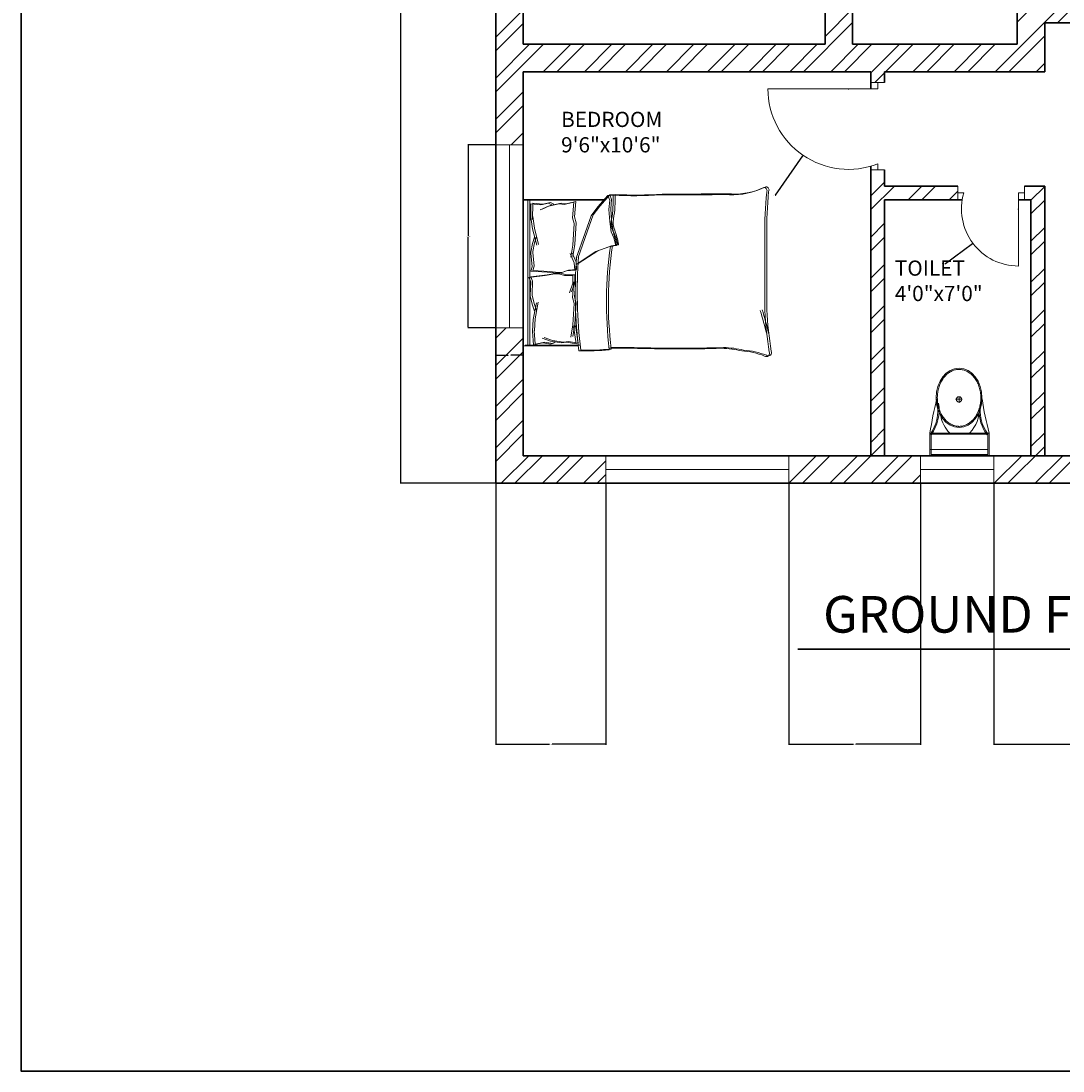
# Model space of a CAD drawing. Units: inches. Extents: x 1955 to 3324, y 980 to 3129.
# Tile 1 of 11: x 1955 to 2296, y 1704 to 2048. Entities that reach past the tile are written whole.
import ezdxf

# ---------------------------------------------------------------- set-up
doc = ezdxf.new("R2010")
doc.units = ezdxf.units.IN
for name, color, linetype, lineweight in [('A-ANNO-DIMS', 2, 'Continuous', 18), ('A-ANNO-TITL', 7, 'Continuous', 35), ('A-ANNO-TTLB', 7, 'Continuous', 35), ('A-AREA-IDEN', 7, 'Continuous', 18), ('A-DOOR', 3, 'Continuous', 18), ('A-FLOR-FIXT', 9, 'Continuous', 18), ('A-FURN', 8, 'Continuous', 18), ('A-GLAZ', 4, 'Continuous', 18), ('A-WALL', 7, 'Continuous', 35), ('A-WALL-PATT', 252, 'Continuous', 13)]:
    doc.layers.add(name, color=color, linetype=linetype, lineweight=lineweight)
doc.styles.get("Standard").update_dxf_attribs({"font": 'arial.ttf'})
doc.dimstyles.get("Standard").update_dxf_attribs({"dimtxt": 0.18, "dimasz": 0.18, "dimexe": 0.18, "dimexo": 0.0625, "dimgap": 0.09, "dimtad": 0, "dimtih": 1, "dimtoh": 1, "dimdec": 4, "dimzin": 0, "dimdsep": 46, "dimtxsty": 'Standard', "dimcen": 0.09, "dimadec": 0, "dimazin": 0, "dimtfac": 1, "dimtdec": 4, "dimtofl": 0, "dimtmove": 0, "dimatfit": 3, "dimfxl": 1, "dimtolj": 1, "dimtzin": 0, "dimarcsym": 0})

# ---------------------------------------------------------------- blocks, each defined once
blk = doc.blocks.new('A$C31115884')
for p, q in [((283.1, 497.7), (223.4, 497.7)), ((257.5, 466.4), (257.5, 523.2)), ((0, 200), (0, 0)), ((520, 200), (0, 200)), ((10, 190), (10, 10)), ((510, 190), (10, 190)), ((510, 10), (510, 190)), ((520, 0), (520, 200)), ((510, 54.5), (0, 54.5)), ((10, 10), (510, 10)), ((0, 0), (520, 0))]:
    blk.add_line(p, q)
blk.add_circle((255.6, 496.4), 23.6)
for centre, radius, start, end in [((2777.7, -204.6), 2807, 165.4549, 171.71327), ((-294.5, 403.3), 364.7, 324.20913, 9.34987), ((-294.5, 403.3), 374.7, 324.20913, 9.34987), ((805.8, 403.3), 364.7, 170.65013, 215.79087), ((3237, 905), 2807, 188.28673, 194.5451), ((139.5, 406.2), 293.5, 315.84364, 2.65635), ((805.8, 403.3), 374.7, 179.20365, 215.79087), ((383.6, 406.2), 293.5, 190.27735, 224.15636)]:
    blk.add_arc(centre, radius, start, end)
blk.add_ellipse((256.2, 509.9), major_axis=(0, -260.7), ratio=0.772727)
blk.add_open_spline([(256.2, 259.2), (263.1, 259.2), (270, 259.7), (287.8, 262.3), (298.7, 265.1), (319.9, 273.1), (330.2, 278.4), (350.1, 291.1), (359.7, 298.7), (377.7, 315.9), (386.2, 325.5), (401.7, 346.6), (408.8, 358.1), (421.3, 382.5), (426.8, 395.5), (435.9, 422.4), (439.5, 436.4), (444.8, 465.1), (446.5, 479.7), (447.9, 509.2), (447.6, 524), (445, 553.3), (442.7, 567.8), (436.3, 596), (432.1, 609.7), (421.9, 636), (416, 648.6), (402.5, 672.1), (395, 683), (378.6, 703), (369.8, 712.1), (351.1, 728), (341.3, 734.8), (320.9, 746.2), (310.4, 750.7), (288.9, 757.3), (278, 759.4), (256, 761), (245, 760.6), (223.1, 757.2), (212.3, 754.3), (191.1, 746.1), (180.8, 740.7), (160.9, 727.8), (151.4, 720.1), (133.5, 702.7), (125.1, 693), (109.6, 671.7), (102.6, 660.2), (90.2, 635.7), (84.9, 622.7), (76, 595.6), (72.4, 581.6), (67.2, 552.9), (65.6, 538.2), (64.4, 508.8), (64.8, 494), (67.5, 464.7), (69.9, 450.2), (76.6, 422), (80.8, 408.3), (91.1, 382.2), (97.2, 369.7), (110.8, 346.3), (118.4, 335.4), (134.8, 315.6), (143.7, 306.7), (162.4, 290.9), (172.3, 284.2), (192.8, 273), (203.3, 268.6), (224.8, 262.2), (235.8, 260.2), (249.9, 259.3), (253, 259.2), (256.2, 259.2)], degree=3, knots=[0, 0, 0, 0, 0.110105, 0.110105, 0.285049, 0.285049, 0.459994, 0.459994, 0.634938, 0.634938, 0.809882, 0.809882, 0.984827, 0.984827, 1.159771, 1.159771, 1.334715, 1.334715, 1.50966, 1.50966, 1.684604, 1.684604, 1.859549, 1.859549, 2.034493, 2.034493, 2.209437, 2.209437, 2.384382, 2.384382, 2.559326, 2.559326, 2.73427, 2.73427, 2.909215, 2.909215, 3.084159, 3.084159, 3.259103, 3.259103, 3.434048, 3.434048, 3.608992, 3.608992, 3.783936, 3.783936, 3.958881, 3.958881, 4.133825, 4.133825, 4.30877, 4.30877, 4.483714, 4.483714, 4.658658, 4.658658, 4.833603, 4.833603, 5.008547, 5.008547, 5.183491, 5.183491, 5.358436, 5.358436, 5.53338, 5.53338, 5.708324, 5.708324, 5.883269, 5.883269, 6.058213, 6.058213, 6.233158, 6.233158, 6.283185, 6.283185, 6.283185, 6.283185])
blk = doc.blocks.new('BED-WITH-PILLOWS')
for p, q in [((3.48, 63.33), (3.48, 81.44)), ((3.48, 63.33), (3.48, 81.44)), ((51.27, 81.44), (3.48, 81.44)), ((3.48, 79.91), (51.27, 79.91)), ((3.48, 79.91), (51.27, 79.91)), ((3.7, 62.69), (3.7, 80.8)), ((3.7, 62.69), (3.7, 80.8)), ((3.7, 79.27), (51.49, 79.27)), ((3.7, 79.27), (51.49, 79.27)), ((24.54, 78.99), (25.98, 79.57)), ((24.54, 78.99), (25.98, 79.57)), ((25.98, 79.57), (26.56, 74.22)), ((25.98, 79.57), (26.56, 74.22)), ((51.27, 81.44), (51.27, 54.83)), ((51.27, 81.44), (51.27, 54.83)), ((51.27, 81.44), (51.49, 81.44)), ((51.49, 81.44), (51.49, 80.8)), ((51.49, 80.8), (51.49, 54.19)), ((51.49, 80.8), (51.49, 54.19)), ((3.89, 78.13), (4.47, 74.95)), ((3.9, 78.11), (8.18, 78.43)), ((3.9, 78.11), (8.18, 78.43)), ((3.9, 78.13), (4.47, 74.95)), ((4.12, 77.49), (4.7, 74.31)), ((4.12, 77.49), (4.7, 74.31)), ((4.13, 77.47), (8.41, 77.8)), ((4.13, 77.47), (8.41, 77.8)), ((8.18, 78.43), (8.29, 78.42)), ((8.18, 78.43), (8.29, 78.42)), ((8.29, 78.42), (12.11, 78.13)), ((8.29, 78.42), (12.11, 78.13)), ((8.41, 77.8), (8.51, 77.78)), ((8.41, 77.8), (8.51, 77.78)), ((8.51, 77.78), (12.34, 77.49)), ((8.51, 77.78), (12.34, 77.49)), ((12.11, 78.13), (17.6, 77.12)), ((12.11, 78.13), (17.6, 77.12)), ((12.34, 77.49), (17.83, 76.48)), ((12.34, 77.49), (17.83, 76.48)), ((14.86, 77.69), (16.88, 78.42)), ((14.86, 77.69), (16.88, 78.42)), ((15.08, 77.05), (17.11, 77.78)), ((15.08, 77.05), (17.11, 77.78)), ((16.88, 78.42), (19.77, 79.14)), ((16.88, 78.42), (19.77, 79.14)), ((17.11, 77.78), (20, 78.5)), ((17.11, 77.78), (20, 78.5)), ((19.77, 79.14), (20.09, 79.14)), ((19.77, 79.14), (20.09, 79.14)), ((20, 78.5), (20.32, 78.5)), ((20, 78.5), (20.32, 78.5)), ((20.09, 79.14), (24.54, 78.99)), ((20.09, 79.14), (24.54, 78.99)), ((20.32, 78.5), (24.77, 78.36)), ((20.32, 78.5), (24.77, 78.36)), ((24.77, 78.36), (26.21, 78.93)), ((24.77, 78.36), (26.21, 78.93)), ((26.21, 78.93), (26.79, 73.58)), ((26.21, 78.93), (26.79, 73.58)), ((27.98, 78.95), (27.73, 73.58)), ((27.98, 78.95), (27.73, 73.58)), ((28.21, 78.31), (27.96, 72.94)), ((28.21, 78.31), (27.96, 72.94)), ((29.46, 78.46), (27.98, 78.95)), ((29.46, 78.46), (27.98, 78.95)), ((29.68, 77.83), (28.21, 78.31)), ((29.68, 77.83), (28.21, 78.31)), ((33.88, 78.89), (29.46, 78.46)), ((33.88, 78.89), (29.46, 78.46)), ((34.11, 78.25), (29.68, 77.83)), ((34.11, 78.25), (29.68, 77.83)), ((34.21, 78.91), (33.88, 78.89)), ((34.2, 78.91), (33.88, 78.89)), ((34.43, 78.27), (34.11, 78.25)), ((34.43, 78.27), (34.11, 78.25)), ((37.14, 78.36), (34.2, 78.91)), ((37.14, 78.36), (34.21, 78.91)), ((37.36, 77.73), (34.43, 78.27)), ((37.36, 77.73), (34.43, 78.27)), ((41.91, 78.37), (36.5, 77.02)), ((41.91, 78.37), (36.5, 77.02)), ((42.14, 77.73), (36.72, 76.38)), ((42.14, 77.73), (36.72, 76.38)), ((39.2, 77.77), (37.14, 78.36)), ((39.2, 77.77), (37.14, 78.36)), ((39.43, 77.13), (37.36, 77.73)), ((39.43, 77.13), (37.36, 77.73)), ((45.71, 78.9), (41.91, 78.37)), ((45.71, 78.9), (41.91, 78.37)), ((45.94, 78.26), (42.14, 77.73)), ((45.94, 78.26), (42.14, 77.73)), ((50.11, 78.89), (44.71, 78.98)), ((44.71, 78.98), (45.71, 78.9)), ((50.11, 78.89), (44.71, 78.98)), ((44.71, 78.98), (45.71, 78.9)), ((50.34, 78.25), (44.94, 78.34)), ((44.94, 78.34), (45.94, 78.26)), ((50.34, 78.25), (44.94, 78.34)), ((44.94, 78.34), (45.94, 78.26)), ((49.31, 73.19), (48.13, 75.86)), ((49.31, 73.19), (48.13, 75.86)), ((50.11, 78.89), (49.73, 75.68)), ((50.11, 78.89), (49.73, 75.68)), ((50.34, 78.25), (49.96, 75.04)), ((50.34, 78.25), (49.96, 75.04)), ((4.47, 74.95), (4.04, 72.34)), ((4.47, 74.95), (4.04, 72.34)), ((4.04, 72.34), (4.62, 71.33)), ((4.04, 72.34), (4.62, 71.33)), ((4.7, 74.31), (4.27, 71.7)), ((4.7, 74.31), (4.27, 71.7)), ((4.47, 68.87), (5.05, 72.49)), ((4.47, 68.87), (5.05, 72.49)), ((5.05, 72.49), (6.06, 75.24)), ((5.05, 72.49), (6.06, 75.24)), ((5.28, 71.85), (6.29, 74.6)), ((5.28, 71.85), (6.29, 74.6)), ((26.56, 74.22), (27.14, 71.04)), ((26.56, 74.22), (27.14, 71.04)), ((26.79, 73.58), (27.37, 70.4)), ((26.79, 73.58), (27.37, 70.4)), ((27.73, 73.58), (27.36, 70.37)), ((27.73, 73.58), (27.36, 70.37)), ((27.96, 72.94), (27.58, 69.73)), ((27.96, 72.94), (27.58, 69.73)), ((49.54, 72.55), (48.36, 75.23)), ((49.54, 72.55), (48.36, 75.23)), ((50.11, 69.61), (49.31, 73.19)), ((50.11, 69.61), (49.31, 73.19)), ((50.34, 68.98), (49.54, 72.55)), ((50.34, 68.98), (49.54, 72.55)), ((49.73, 75.68), (50.33, 73.11)), ((49.73, 75.68), (50.33, 73.11)), ((50.33, 73.11), (49.81, 72.06)), ((50.33, 73.11), (49.82, 72.06)), ((49.96, 75.04), (50.56, 72.47)), ((49.96, 75.04), (50.56, 72.47)), ((50.56, 72.47), (50.04, 71.42)), ((50.56, 72.47), (50.04, 71.42)), ((4.27, 71.7), (4.85, 70.69)), ((4.27, 71.7), (4.85, 70.69)), ((4.7, 68.23), (5.28, 71.85)), ((4.7, 68.23), (5.28, 71.85)), ((27.14, 69.74), (26.56, 67.86)), ((27.14, 69.74), (26.56, 67.86)), ((27.37, 69.1), (26.79, 67.22)), ((27.37, 69.1), (26.79, 67.22)), ((27.14, 71.04), (27.14, 69.74)), ((27.14, 71.04), (27.14, 69.74)), ((27.36, 70.37), (27.44, 69.07)), ((27.36, 70.37), (27.44, 69.07)), ((27.37, 70.4), (27.37, 69.1)), ((27.37, 70.4), (27.37, 69.1)), ((27.44, 69.07), (28.13, 67.23)), ((27.44, 69.07), (28.13, 67.23)), ((27.58, 69.73), (27.66, 68.43)), ((27.58, 69.73), (27.66, 68.43)), ((49.92, 68.01), (50.11, 69.61)), ((49.92, 68.01), (50.11, 69.61)), ((50.15, 67.37), (50.34, 68.98)), ((50.15, 67.37), (50.34, 68.98)), ((4.18, 64.1), (4.76, 67.28)), ((4.18, 64.1), (4.76, 67.28)), ((4.41, 63.46), (4.99, 66.64)), ((4.41, 63.46), (4.99, 66.64)), ((4.76, 67.28), (4.47, 68.87)), ((4.76, 67.28), (4.47, 68.87)), ((4.99, 66.64), (4.7, 68.23)), ((4.99, 66.64), (4.7, 68.23)), ((6.38, 65.81), (10.41, 65.15)), ((6.38, 65.81), (10.41, 65.15)), ((24.1, 65.18), (20.96, 66.27)), ((24.1, 65.18), (20.96, 66.27)), ((24.33, 64.54), (21.19, 65.63)), ((24.33, 64.54), (21.19, 65.63)), ((26.56, 67.86), (26.56, 65.18)), ((26.56, 67.86), (26.56, 65.18)), ((26.79, 67.22), (26.79, 64.54)), ((26.79, 67.22), (26.79, 64.54)), ((27.66, 68.43), (28.36, 66.59)), ((27.66, 68.43), (28.36, 66.59)), ((28.13, 67.23), (28.3, 64.55)), ((28.13, 67.23), (28.3, 64.55)), ((28.36, 66.59), (28.53, 63.91)), ((28.36, 66.59), (28.53, 63.91)), ((30.75, 64.7), (33.82, 65.99)), ((30.75, 64.7), (33.82, 65.99)), ((32.56, 65.81), (36.6, 65.15)), ((32.56, 65.81), (36.6, 65.15)), ((50.7, 64.87), (49.92, 68.01)), ((50.7, 64.87), (49.92, 68.01)), ((50.93, 64.23), (50.15, 67.37)), ((50.93, 64.23), (50.15, 67.37)), ((9.28, 64.83), (4.18, 64.1)), ((9.28, 64.83), (4.18, 64.1)), ((9.51, 64.19), (4.41, 63.46)), ((9.51, 64.19), (4.41, 63.46)), ((6.61, 65.18), (10.64, 64.51)), ((6.61, 65.18), (10.64, 64.51)), ((10.41, 65.15), (9.28, 64.83)), ((10.41, 65.15), (9.28, 64.83)), ((10.64, 64.51), (9.51, 64.19)), ((10.64, 64.51), (9.51, 64.19)), ((10.41, 65.15), (17.42, 64.72)), ((10.41, 65.15), (17.42, 64.72)), ((10.64, 64.51), (17.65, 64.08)), ((10.64, 64.51), (17.65, 64.08)), ((17.42, 64.72), (19.38, 65.27)), ((17.42, 64.72), (19.38, 65.27)), ((17.65, 64.08), (19.61, 64.63)), ((17.65, 64.08), (19.61, 64.63)), ((19.38, 65.27), (24.52, 64.87)), ((19.38, 65.27), (24.52, 64.87)), ((19.61, 64.63), (24.74, 64.23)), ((19.61, 64.63), (24.74, 64.23)), ((26.56, 65.18), (24.1, 65.18)), ((26.56, 65.18), (24.1, 65.18)), ((26.79, 64.54), (24.33, 64.54)), ((26.79, 64.54), (24.33, 64.54)), ((28.3, 64.55), (30.75, 64.7)), ((28.3, 64.55), (30.75, 64.7)), ((28.53, 63.91), (30.98, 64.06)), ((28.53, 63.91), (30.98, 64.06)), ((30.26, 64.06), (34.45, 57.57)), ((30.26, 64.06), (34.45, 57.57)), ((30.49, 63.42), (34.68, 56.93)), ((30.49, 63.42), (34.68, 56.93)), ((30.98, 64.06), (34.05, 65.35)), ((30.98, 64.06), (34.05, 65.35)), ((40.64, 61.13), (32.31, 64.06)), ((40.64, 61.13), (32.31, 64.06)), ((40.87, 60.49), (32.53, 63.42)), ((40.87, 60.49), (32.54, 63.42)), ((32.79, 65.18), (36.83, 64.51)), ((32.79, 65.18), (36.82, 64.51)), ((36.6, 65.15), (43.61, 64.72)), ((36.6, 65.15), (43.61, 64.72)), ((36.82, 64.51), (43.83, 64.08)), ((36.83, 64.51), (43.84, 64.08)), ((43.61, 64.72), (45.57, 65.27)), ((43.61, 64.72), (45.57, 65.27)), ((43.83, 64.08), (45.8, 64.63)), ((43.84, 64.08), (45.8, 64.63)), ((45.57, 65.27), (50.7, 64.87)), ((45.57, 65.27), (50.7, 64.87)), ((45.8, 64.63), (50.93, 64.23)), ((45.8, 64.63), (50.93, 64.23)), ((46.22, 59.11), (40.64, 61.13)), ((46.22, 59.11), (40.64, 61.13)), ((46.45, 58.48), (40.87, 60.49)), ((46.45, 58.48), (40.87, 60.49)), ((49.16, 56.95), (46.22, 59.11)), ((49.16, 56.95), (46.22, 59.11)), ((34.45, 57.57), (36.15, 53.08)), ((34.45, 57.57), (36.15, 53.08)), ((34.68, 56.93), (36.38, 52.44)), ((34.68, 56.93), (36.38, 52.44)), ((49.39, 56.31), (46.45, 58.48)), ((49.39, 56.31), (46.45, 58.48)), ((52.87, 53.7), (49.16, 56.95)), ((52.87, 53.7), (49.16, 56.95)), ((53.1, 53.06), (49.39, 56.31)), ((53.1, 53.06), (49.39, 56.31)), ((36.15, 53.08), (36.46, 51.07)), ((36.15, 53.08), (36.46, 51.07)), ((36.38, 52.44), (36.69, 50.43)), ((36.38, 52.44), (36.69, 50.43)), ((36.46, 51.07), (38.94, 51.69)), ((36.46, 51.07), (38.94, 51.69)), ((38.94, 51.69), (40.95, 52.61)), ((38.94, 51.69), (40.95, 52.61)), ((39.17, 51.05), (41.18, 51.97)), ((39.17, 51.05), (41.18, 51.97)), ((40.95, 52.61), (44.36, 53.08)), ((40.95, 52.61), (44.36, 53.08)), ((41.18, 51.97), (44.59, 52.44)), ((41.18, 51.97), (44.59, 52.44)), ((44.36, 53.08), (48.23, 53.39)), ((44.36, 53.08), (48.23, 53.39)), ((44.59, 52.44), (48.46, 52.75)), ((44.59, 52.44), (48.46, 52.75)), ((48.23, 53.39), (51.33, 53.08)), ((48.23, 53.39), (51.33, 53.08)), ((48.46, 52.75), (51.56, 52.44)), ((48.46, 52.75), (51.56, 52.44)), ((51.33, 53.08), (52.87, 53.7)), ((51.33, 53.08), (52.87, 53.7)), ((51.56, 52.44), (53.1, 53.06)), ((51.56, 52.44), (53.1, 53.06)), ((52.95, 51.95), (52.87, 53.7, 3.87)), ((52.95, 51.95), (52.87, 53.7, 3.87)), ((53.18, 51.31), (53.1, 53.06, 3.87)), ((53.18, 51.31), (53.1, 53.06, 3.87)), ((36.69, 50.43), (39.17, 51.05)), ((36.69, 50.43), (39.17, 51.05)), ((15.06, 2.2), (39.68, 2.2)), ((15.06, 2.2), (39.68, 2.2)), ((15.29, 1.56), (39.91, 1.56)), ((15.29, 1.56), (39.91, 1.56))]:
    blk.add_line(p, q)
for centre, radius, start, end in [((85.16, 61.35), 83.31, 178.7218, 185.604), ((85.16, 61.35), 83.31, 178.7218, 185.604), ((21.36, -100.61), 164.97, 86.0865, 96.7821), ((21.36, -100.61), 164.97, 86.0865, 96.7821), ((85.39, 60.71), 83.31, 178.7218, 185.604), ((85.39, 60.71), 83.31, 178.7218, 185.604), ((21.59, -101.25), 164.97, 86.0865, 96.7821), ((21.59, -101.25), 164.97, 86.0865, 96.7821), ((17.76, -74.87), 129.02, 81.7845, 96.9006), ((17.76, -74.87), 129.02, 81.7845, 96.9006), ((17.98, -75.51), 129.02, 81.7845, 96.9006), ((17.98, -75.51), 129.02, 81.7845, 96.9006), ((-167.31, 50.27), 170.11, 358.4762, 1.0082), ((-167.31, 50.27), 170.11, 358.4762, 1.0082), ((-167.08, 49.63), 170.11, 358.4762, 1.0082), ((-167.08, 49.63), 170.11, 358.4762, 1.0082), ((31.15, 79.96), 29.65, 280.6617, 289.8806), ((31.15, 79.96), 29.65, 280.6617, 289.8806), ((43.74, 46.38), 6.22, 78.6608, 113.7384), ((43.74, 46.38), 6.22, 78.6608, 113.7384), ((43.97, 45.74), 6.22, 78.6608, 113.7384), ((43.97, 45.74), 6.22, 78.6608, 113.7384), ((51.33, 88.1), 36.18, 259.8763, 272.5657), ((51.33, 88.1), 36.18, 259.8763, 272.5657), ((51.56, 87.46), 36.18, 259.8763, 272.5657), ((51.56, 87.46), 36.18, 259.8763, 272.5657), ((182.27, 45.13), 129.5, 176.9791, 183.8365), ((182.27, 45.13), 129.5, 176.9791, 183.8365), ((36.64, 51), 0.185, 160.2464, 271.1377), ((36.64, 51), 0.185, 160.2464, 271.1377), ((36.87, 50.36), 0.185, 160.2464, 271.1377), ((36.86, 50.36), 0.185, 160.2464, 271.1377), ((31.38, 79.32), 29.65, 280.6617, 289.8806), ((31.38, 79.32), 29.65, 280.6617, 289.8806), ((182.49, 44.49), 129.5, 176.9791, 183.8365), ((182.49, 44.49), 129.5, 176.9791, 183.8365), ((484.82, 30.83), 482.31, 178.2277, 181.7185), ((484.82, 30.83), 482.31, 178.2277, 181.7185), ((485.05, 30.19), 482.31, 178.2277, 181.7185), ((485.05, 30.19), 482.31, 178.2277, 181.7185), ((-4508.74, 13.62), 4561.86, 0.00217, 0.28689), ((-4508.74, 13.62), 4561.86, 0.00217, 0.28689), ((-4508.51, 12.98), 4561.86, 0.00217, 0.28689), ((-4508.51, 12.98), 4561.86, 0.00217, 0.28689), ((-26.9, 16.93), 29.63, 346.0648, 358.9113), ((-26.9, 16.93), 29.63, 346.0648, 358.9113), ((-26.67, 16.29), 29.63, 346.0648, 358.9113), ((-26.67, 16.29), 29.63, 346.0648, 358.9113), ((76.16, 12.78), 23.07, 177.4714, 206.4681), ((76.16, 12.78), 23.07, 177.4714, 206.4681), ((76.39, 12.14), 23.07, 177.4714, 206.4681), ((76.39, 12.14), 23.07, 177.4714, 206.4681), ((-21.66, 11.17), 23.56, 337.9751, 356.652), ((-21.66, 11.17), 23.56, 337.9751, 356.652), ((-21.43, 10.53), 23.56, 337.9751, 356.652), ((-21.43, 10.53), 23.56, 337.9751, 356.652), ((-17.22, 105.16), 106.46, 283.3832, 287.7053), ((-17.22, 105.16), 106.46, 283.3832, 287.7053), ((1.09, 1.73), 1.09, 146.1736, 293.4781), ((1.09, 1.73), 1.09, 146.1736, 293.4781), ((1.32, 1.09), 1.09, 146.1736, 293.4781), ((1.32, 1.09), 1.09, 146.1736, 293.4781), ((21.43, -119.39), 121.76, 92.9958, 99.4091), ((21.43, -119.39), 121.76, 92.9958, 99.4091), ((21.66, -120.03), 121.76, 92.9958, 99.4091), ((21.66, -120.03), 121.76, 92.9958, 99.4091), ((-16.99, 104.52), 106.46, 283.3832, 287.7053), ((-16.99, 104.52), 106.46, 283.3832, 287.7053), ((41.15, -130.83), 133.04, 84.4998, 90.6351), ((41.15, -130.83), 133.04, 84.4998, 90.6351), ((41.38, -131.47), 133.04, 84.4998, 90.6351), ((41.38, -131.47), 133.04, 84.4998, 90.6351), ((54.41, 2.57), 1.1, 242.6588, 356.02), ((54.41, 2.57), 1.1, 242.6588, 356.02), ((54.64, 1.93), 1.1, 242.6588, 356.02), ((54.64, 1.93), 1.1, 242.6588, 356.02)]:
    blk.add_arc(centre, radius, start, end)
blk = doc.blocks.new('DOOR-BED-S')
for p, q in [((38.25, 28.66), (33.75, 28.66)), ((33.75, 28.66), (36, 28.66)), ((36, 28.66), (36, 26.66)), ((36, 26.66), (0, 26.66)), ((36, 0), (36, 2)), ((33.75, 0), (38.25, 0)), ((38.25, 0), (36, 0))]:
    blk.add_line(p, q)
blk.add_arc((26.45, 26.66), 26.45, 180, 291.1718)
blk = doc.blocks.new('DOOR-WC-S')
for p, q in [((0, 21.75), (0, 26.25)), ((0, 26.25), (0, 24)), ((21.9, 21.75), (21.9, 26.25)), ((21.9, 26.25), (21.9, 24)), ((0, 24), (2, 24)), ((21.9, 24), (19.9, 24)), ((19.9, 24), (19.9, 0))]:
    blk.add_line(p, q)
blk.add_arc((19.9, 18.68), 18.68, 163.4391, 270)
blk = doc.blocks.new('WIN-PLAN-60-A')
for p, q in [((0, 60), (9, 60)), ((9, 60), (4.5, 60)), ((4.5, 60), (4.5, 0)), ((4.5, 0), (0, 0)), ((0, 0), (9, 0))]:
    blk.add_line(p, q)
blk = doc.blocks.new('WIN-PLAN-60-B')
for p, q in [((0, 0), (0, 9)), ((0, 9), (0, 4.5)), ((60, 4.5), (60, 9)), ((60, 9), (60, 0)), ((0, 4.5), (60, 4.5))]:
    blk.add_line(p, q)
blk = doc.blocks.new('WIN-PLAN-24-A')
for p, q in [((0, 9), (0, 0)), ((24, 4.5), (24, 9)), ((24, 9), (24, 0)), ((0, 0), (0, 4.5)), ((0, 4.5), (24, 4.5))]:
    blk.add_line(p, q)
blk = doc.blocks.new('*D33')
at = {"layer": 'A-ANNO-DIMS', "color": 0, "lineweight": -2, "transparency": 16777216}
for p, q in [((2110.15, 2007.51), (2101.03, 2007.51)), ((2101.21, 2007.33), (2101.21, 1977.7)), ((2101.21, 1947.69), (2101.21, 1977.33)), ((2110.15, 1947.51), (2101.03, 1947.51))]:
    blk.add_line(p, q, dxfattribs=at)
at = {"layer": 'A-ANNO-DIMS', "color": 0, "transparency": 16777216}
for points in [[(2101.18, 2007.33), (2101.24, 2007.33), (2101.21, 2007.51)], [(2101.18, 1947.69), (2101.24, 1947.69), (2101.21, 1947.51)]]:
    blk.add_solid(points, dxfattribs=at)
at = {"layer": 'Defpoints', "color": 0, "transparency": 16777216}
for p in [(2110.21, 2007.51), (2101.21, 1947.51), (2110.21, 1947.51)]:
    blk.add_point(p, dxfattribs=at)
at = {"layer": 'A-ANNO-DIMS', "color": 0, "transparency": 16777216, "insert": (2101.21, 1977.51), "char_height": 0.18, "attachment_point": 5}
blk.add_mtext('\\A1;WIN. 60 TYP.', dxfattribs=at)
blk = doc.blocks.new('*D34')
at = {"layer": 'A-ANNO-DIMS', "color": 0, "lineweight": -2, "transparency": 16777216}
for p, q in [((2110.21, 1947.45), (2110.21, 1938.33)), ((2119.21, 1947.45), (2119.21, 1938.33)), ((2110.39, 1938.51), (2114.25, 1938.51)), ((2119.03, 1938.51), (2115.17, 1938.51))]:
    blk.add_line(p, q, dxfattribs=at)
at = {"layer": 'A-ANNO-DIMS', "color": 0, "transparency": 16777216}
for points in [[(2110.39, 1938.54), (2110.39, 1938.48), (2110.21, 1938.51)], [(2119.03, 1938.54), (2119.03, 1938.48), (2119.21, 1938.51)]]:
    blk.add_solid(points, dxfattribs=at)
at = {"layer": 'Defpoints', "color": 0, "transparency": 16777216}
for p in [(2110.21, 1947.51), (2119.21, 1947.51), (2119.21, 1938.51)]:
    blk.add_point(p, dxfattribs=at)
at = {"layer": 'A-ANNO-DIMS', "color": 0, "transparency": 16777216, "insert": (2114.71, 1938.51), "char_height": 0.18, "attachment_point": 5}
blk.add_mtext('\\A1;9 TYP.', dxfattribs=at)
blk = doc.blocks.new('*D92')
at = {"layer": 'A-ANNO-DIMS', "color": 0, "lineweight": -2, "transparency": 16777216}
for p, q in [((2110.15, 2456.5), (2078.88, 2456.5)), ((2079.06, 2456.32), (2079.06, 2176.69)), ((2079.06, 1896.68), (2079.06, 2176.32)), ((2110.15, 1896.5), (2078.88, 1896.5))]:
    blk.add_line(p, q, dxfattribs=at)
at = {"layer": 'A-ANNO-DIMS', "color": 0, "transparency": 16777216}
for points in [[(2079.03, 2456.32), (2079.09, 2456.32), (2079.06, 2456.5)], [(2079.03, 1896.68), (2079.09, 1896.68), (2079.06, 1896.5)]]:
    blk.add_solid(points, dxfattribs=at)
at = {"layer": 'Defpoints', "color": 0, "transparency": 16777216}
for p in [(2079.06, 2456.5), (2110.21, 2456.5), (2110.21, 1896.5)]:
    blk.add_point(p, dxfattribs=at)
at = {"layer": 'A-ANNO-DIMS', "color": 0, "transparency": 16777216, "insert": (2079.06, 2176.5), "char_height": 0.18, "attachment_point": 5}
blk.add_mtext('\\A1;560', dxfattribs=at)
blk = doc.blocks.new('*D107')
at = {"layer": 'A-ANNO-DIMS', "color": 0, "lineweight": -2, "transparency": 16777216}
for p, q in [((2110.21, 1896.44), (2110.21, 1810.7)), ((2146.36, 1896.44), (2146.36, 1810.7)), ((2110.39, 1810.88), (2127.89, 1810.88)), ((2146.18, 1810.88), (2128.68, 1810.88))]:
    blk.add_line(p, q, dxfattribs=at)
at = {"layer": 'A-ANNO-DIMS', "color": 0, "transparency": 16777216}
for points in [[(2110.39, 1810.91), (2110.39, 1810.85), (2110.21, 1810.88)], [(2146.18, 1810.91), (2146.18, 1810.85), (2146.36, 1810.88)]]:
    blk.add_solid(points, dxfattribs=at)
at = {"layer": 'Defpoints', "color": 0, "transparency": 16777216}
for p in [(2110.21, 1896.5), (2146.36, 1896.5), (2146.36, 1810.88)]:
    blk.add_point(p, dxfattribs=at)
at = {"layer": 'A-ANNO-DIMS', "color": 0, "transparency": 16777216, "insert": (2128.29, 1810.88), "char_height": 0.18, "attachment_point": 5}
blk.add_mtext('\\A1;36.15', dxfattribs=at)
blk = doc.blocks.new('*D108')
at = {"layer": 'A-ANNO-DIMS', "color": 0, "lineweight": -2, "transparency": 16777216}
for p, q in [((2206.36, 1896.44), (2206.36, 1810.7)), ((2249.49, 1896.44), (2249.49, 1810.7)), ((2206.54, 1810.88), (2227.53, 1810.88)), ((2249.31, 1810.88), (2228.32, 1810.88))]:
    blk.add_line(p, q, dxfattribs=at)
at = {"layer": 'A-ANNO-DIMS', "color": 0, "transparency": 16777216}
for points in [[(2206.54, 1810.91), (2206.54, 1810.85), (2206.36, 1810.88)], [(2249.31, 1810.91), (2249.31, 1810.85), (2249.49, 1810.88)]]:
    blk.add_solid(points, dxfattribs=at)
at = {"layer": 'Defpoints', "color": 0, "transparency": 16777216}
for p in [(2206.36, 1896.5), (2249.49, 1896.5), (2249.49, 1810.88)]:
    blk.add_point(p, dxfattribs=at)
at = {"layer": 'A-ANNO-DIMS', "color": 0, "transparency": 16777216, "insert": (2227.93, 1810.88), "char_height": 0.18, "attachment_point": 5}
blk.add_mtext('\\A1;43.13', dxfattribs=at)
blk = doc.blocks.new('*D109')
at = {"layer": 'A-ANNO-DIMS', "color": 0, "lineweight": -2, "transparency": 16777216}
for p, q in [((2273.49, 1896.44), (2273.49, 1810.7)), ((2342.7, 1896.44), (2342.7, 1810.7)), ((2273.67, 1810.88), (2307.72, 1810.88)), ((2342.52, 1810.88), (2308.47, 1810.88))]:
    blk.add_line(p, q, dxfattribs=at)
at = {"layer": 'A-ANNO-DIMS', "color": 0, "transparency": 16777216}
for points in [[(2273.67, 1810.91), (2273.67, 1810.85), (2273.49, 1810.88)], [(2342.52, 1810.91), (2342.52, 1810.85), (2342.7, 1810.88)]]:
    blk.add_solid(points, dxfattribs=at)
at = {"layer": 'Defpoints', "color": 0, "transparency": 16777216}
for p in [(2273.49, 1896.5), (2342.7, 1896.5), (2342.7, 1810.88)]:
    blk.add_point(p, dxfattribs=at)
at = {"layer": 'A-ANNO-DIMS', "color": 0, "transparency": 16777216, "insert": (2308.09, 1810.88), "char_height": 0.18, "attachment_point": 5}
blk.add_mtext('\\A1;69.21', dxfattribs=at)
blk = doc.blocks.new('*D144')
at = {"layer": 'A-ANNO-DIMS', "color": 0, "lineweight": -2, "transparency": 16777216}
for p, q in [((2225.82, 2025.93), (2226, 2025.93)), ((2225.91, 2025.84), (2225.91, 2026.02)), ((2201.99, 1991.02), (2210.86, 2003.96)), ((2201.81, 1991.02), (2201.99, 1991.02))]:
    blk.add_line(p, q, dxfattribs=at)
at = {"layer": 'A-ANNO-DIMS', "color": 0, "transparency": 16777216}
blk.add_solid([(2210.83, 2003.98), (2210.88, 2003.94), (2210.96, 2004.11)], dxfattribs=at)
at = {"layer": 'Defpoints', "color": 0, "transparency": 16777216}
for p in [(2225.91, 2025.93), (2210.96, 2004.11)]:
    blk.add_point(p, dxfattribs=at)
at = {"layer": 'A-ANNO-DIMS', "color": 0, "transparency": 16777216, "insert": (2201.33, 1991.02), "char_height": 0.18, "attachment_point": 5}
blk.add_mtext('\\A1;R26.45', dxfattribs=at)
blk = doc.blocks.new('*D146')
at = {"layer": 'A-ANNO-DIMS', "color": 0, "lineweight": -2, "transparency": 16777216}
for p, q in [((2281.52, 1986.43), (2281.7, 1986.43)), ((2281.61, 1986.34), (2281.61, 1986.52)), ((2257.66, 1968.56), (2266.5, 1975.16)), ((2257.48, 1968.56), (2257.66, 1968.56))]:
    blk.add_line(p, q, dxfattribs=at)
at = {"layer": 'A-ANNO-DIMS', "color": 0, "transparency": 16777216}
blk.add_solid([(2266.48, 1975.18), (2266.51, 1975.13), (2266.64, 1975.26)], dxfattribs=at)
at = {"layer": 'Defpoints', "color": 0, "transparency": 16777216}
for p in [(2281.61, 1986.43), (2266.64, 1975.26)]:
    blk.add_point(p, dxfattribs=at)
at = {"layer": 'A-ANNO-DIMS', "color": 0, "transparency": 16777216, "insert": (2256.93, 1968.56), "char_height": 0.18, "attachment_point": 5}
blk.add_mtext('\\A1;R18.677', dxfattribs=at)

msp = doc.modelspace()

# ---------------------------------------------------------------- hatches: boundary and pattern name
at = {"layer": 'A-WALL-PATT'}
h = msp.add_hatch(dxfattribs=at)
h.set_pattern_fill('ANSI32', color=256)
h.paths.add_polyline_path([(2361.4775, 2456.5037), (2270.2755, 2456.5037), (2270.2755, 2447.5037), (2285.7102, 2447.5037), (2285.7102, 2363.5037), (2281.1795, 2363.5037), (2281.1795, 2359.0037), (2290.2102, 2359.0037), (2290.2102, 2447.5037), (2361.4775, 2447.5037), (2361.4775, 2452.0037)])
h.paths.add_polyline_path([(2246.2755, 2456.5037), (2197.6809, 2456.5037), (2197.6809, 2447.5037), (2233.2102, 2447.5037), (2233.2102, 2355.6044), (2237.7102, 2355.6044), (2237.7102, 2447.5037), (2246.2755, 2447.5037)], flags=17)
h.paths.add_polyline_path([(2137.6809, 2456.5037), (2110.2102, 2456.5037), (2110.2102, 2312.5037), (2152.2102, 2312.5037), (2281.2102, 2312.5037), (2281.2102, 2107.6185), (2290.2102, 2107.6185), (2290.2102, 2267.9289), (2329.216, 2267.9289), (2329.216, 2272.4289), (2329.216, 2276.9289), (2290.2102, 2276.9289), (2290.2102, 2321.5037), (2281.2102, 2321.5037), (2119.2102, 2321.5037), (2119.2102, 2447.5037), (2137.6809, 2447.5037)])
h.paths.add_polyline_path([(2515.2102, 2456.5037), (2421.4775, 2456.5037), (2421.4775, 2447.5037), (2506.2102, 2447.5037), (2506.2102, 2415.6626), (2515.2102, 2415.6626)])
h.paths.add_polyline_path([(2515.2102, 2355.6626), (2506.2102, 2355.6626), (2506.2102, 2321.5037), (2424.9282, 2321.5037), (2424.9282, 2312.5037), (2461.2102, 2312.5037), (2470.2102, 2312.5037), (2515.2102, 2312.5037)])
h.paths.add_polyline_path([(2515.2102, 2232.5037), (2470.2102, 2232.5037), (2470.2102, 2237.3759), (2465.7102, 2237.3759), (2461.2102, 2237.3759), (2461.2102, 2232.5037), (2377.2219, 2232.5037), (2377.2219, 2321.5037), (2368.2219, 2321.5037), (2368.2219, 2276.9289), (2359.3802, 2276.9289), (2359.3802, 2272.4289), (2359.3802, 2267.9289), (2368.2219, 2267.9289), (2368.2219, 2223.5037), (2377.2219, 2223.5037), (2461.2102, 2223.5037), (2506.2102, 2223.5037), (2506.2102, 2129.5037), (2461.2102, 2129.5037), (2387.2102, 2129.5037), (2368.2219, 2129.5037), (2368.2219, 2056.4936), (2361.0095, 2056.4936), (2361.0095, 2051.9936), (2361.0095, 2047.4936), (2368.2219, 2047.4936), (2368.2219, 2031.5037), (2377.2219, 2031.5037), (2377.2219, 2120.5037), (2461.2102, 2120.5037), (2461.2102, 2112.7921), (2470.2102, 2112.7921), (2470.2102, 2120.5037), (2515.2102, 2120.5037), (2515.2102, 2129.5037)])
h.paths.add_polyline_path([(2470.2102, 2277.1758), (2461.2102, 2277.1758), (2461.2102, 2272.5037), (2461.2102, 2270.2549), (2470.2102, 2270.2549), (2470.2102, 2272.5037)], flags=17)
h.paths.add_polyline_path([(2515.2102, 2040.5037), (2470.2102, 2040.5037), (2417.8264, 2040.5037), (2417.8264, 2031.5037), (2506.2102, 2031.5037), (2506.2102, 2005.3639), (2515.2102, 2005.3639)])
h.paths.add_polyline_path([(2506.2102, 1905.5037), (2402.6963, 1905.5037), (2402.6963, 1896.5037), (2506.2102, 1896.5037)])
h.paths.add_polyline_path([(2515.2102, 1945.3639), (2506.2102, 1945.3639), (2506.2102, 1905.5037), (2506.2102, 1896.5037), (2515.2102, 1896.5037)])
h.paths.add_polyline_path([(2342.6963, 1901.0037), (2342.6963, 1905.5037), (2273.4892, 1905.5037), (2273.4892, 1896.5037), (2342.6963, 1896.5037)])
h.paths.add_polyline_path([(2290.2102, 1994.0037), (2283.612, 1994.0037), (2283.612, 1991.7537), (2283.612, 1989.5037), (2285.7102, 1989.5037), (2285.7102, 1905.5037), (2290.2102, 1905.5037)])
h.paths.add_polyline_path([(2249.4892, 1905.5037), (2237.7102, 1905.5037), (2206.3617, 1905.5037), (2206.3617, 1896.5037), (2249.4892, 1896.5037), (2249.4892, 1901.0037)])
h.paths.add_polyline_path([(2237.7102, 1989.5037), (2261.7102, 1989.5037), (2261.7102, 1994.0037), (2237.7102, 1994.0037), (2237.7102, 1999.266), (2235.4602, 1999.266), (2233.2102, 1999.266), (2233.2102, 1994.0037), (2233.2102, 1905.5037), (2237.7102, 1905.5037)])
h.paths.add_polyline_path([(2119.2102, 1947.5144), (2110.2102, 1947.5144), (2110.2102, 1896.5037), (2119.2102, 1896.5037), (2146.3617, 1896.5037), (2146.3617, 1901.0037), (2146.3617, 1905.5037), (2119.2102, 1905.5037)])
h.paths.add_polyline_path([(2119.2102, 2068.6379), (2110.2102, 2068.6379), (2110.2102, 2007.5144), (2119.2102, 2007.5144), (2119.2102, 2031.5037), (2233.2102, 2031.5037), (2233.2102, 2027.9287), (2235.4602, 2027.9287), (2237.7102, 2027.9287), (2237.7102, 2031.5037), (2281.2102, 2031.5037), (2290.2102, 2031.5037), (2290.2102, 2047.4936), (2326.409, 2047.4936), (2326.409, 2056.4936), (2290.2102, 2056.4936), (2290.2102, 2071.2722), (2285.7102, 2071.2722), (2281.2102, 2071.2722), (2281.2102, 2040.5037), (2227.2102, 2040.5037), (2227.2102, 2111.2571), (2222.7102, 2111.2571), (2218.2102, 2111.2571), (2218.2102, 2040.5037), (2119.2102, 2040.5037)])
h.paths.add_polyline_path([(2236.9166, 2214.5037), (2161.2102, 2214.5037), (2161.2102, 2221.6488), (2152.2102, 2221.6488), (2152.2102, 2214.5037), (2110.2102, 2214.5037), (2110.2102, 2205.5037), (2131.2394, 2205.5037), (2131.2394, 2198.3478), (2140.2394, 2198.3478), (2140.2394, 2205.5037), (2224.2394, 2205.5037), (2224.2394, 2200.2317), (2228.7394, 2200.2317), (2233.2394, 2200.2317), (2233.2394, 2205.5037), (2236.9166, 2205.5037)], flags=17)
h.paths.add_polyline_path([(2236.9166, 2157.5037), (2233.2394, 2157.5037), (2233.2394, 2178.9172), (2228.7394, 2178.9172), (2224.2394, 2178.9172), (2224.2394, 2157.5037), (2140.2394, 2157.5037), (2140.2394, 2174.3478), (2131.2394, 2174.3478), (2131.2394, 2157.5037), (2110.2102, 2157.5037), (2110.2102, 2128.6379), (2119.2102, 2128.6379), (2119.2102, 2148.5037), (2218.2102, 2148.5037), (2218.2102, 2141.7262), (2222.7102, 2141.7262), (2227.2102, 2141.7262), (2227.2102, 2148.5037), (2236.9166, 2148.5037)], flags=0)
h.paths.add_polyline_path([(3084.7449, 2537.3808), (3212.7954, 2537.3808), (3212.7954, 2555.9271), (3084.7449, 2555.9271)], flags=9)
h.paths.add_polyline_path([(3068.7485, 2853.43), (3169.977, 2853.43), (3169.977, 2871.9764), (3068.7485, 2871.9764)], flags=9)
h.paths.add_polyline_path([(3074.1798, 2918.0252), (3126.4732, 2918.0252), (3126.4732, 2936.5716), (3074.1798, 2936.5716)], flags=9)
h.paths.add_polyline_path([(3073.0928, 2947.3127), (3199.0499, 2947.3127), (3199.0499, 2965.8591), (3073.0928, 2965.8591)], flags=9)
h.paths.add_polyline_path([(2733.8393, 2484.8678), (2879.7915, 2484.8678), (2879.7915, 2521.9606), (2733.8393, 2521.9606)], flags=9)
h.paths.add_polyline_path([(2204.9881, 2482.4168), (2355.1272, 2482.4168), (2355.1272, 2519.5095), (2204.9881, 2519.5095)], flags=9)
h.paths.add_polyline_path([(3062.1429, 2387.2466), (3079.3735, 2387.2466), (3079.3735, 2411.9751), (3062.1429, 2411.9751)], flags=9)
h.paths.add_polyline_path([(2190.1574, 2158.8439), (2219.315, 2158.8439), (2219.315, 2177.5013), (2190.1574, 2177.5013)], flags=25)
h.paths.add_polyline_path([(2213.6766, 1840.7276), (2405.0382, 1840.7276), (2405.0382, 1865.4561), (2213.6766, 1865.4561)], flags=9)
h.paths.add_polyline_path([(2180.5398, 2233.911), (2213.9471, 2233.911), (2213.9471, 2252.5683), (2180.5398, 2252.5683)], flags=25)
h.paths.add_polyline_path([(2134.4484, 2238.3973), (2134.4484, 2274.2807), (2115.791, 2274.2807), (2115.791, 2238.3973)], flags=25)
h.paths.add_polyline_path([(2135.1593, 2122.9991), (2173.7507, 2122.9991), (2173.7507, 2141.6565), (2135.1593, 2141.6565)], flags=25)
h.paths.add_polyline_path([(2129.8822, 2002.1912), (2168.4736, 2002.1912), (2168.4736, 2020.8486), (2129.8822, 2020.8486)], flags=9)
h.paths.add_polyline_path([(2239.6647, 1953.4107), (2268.8973, 1953.4107), (2268.8973, 1972.068), (2239.6647, 1972.068)], flags=9)
h.paths.add_polyline_path([(2352.8562, 1951.2904), (2402.1775, 1951.2904), (2402.1775, 1969.9477), (2352.8562, 1969.9477)], flags=9)
h.paths.add_polyline_path([(2500.1358, 2055.32), (2500.1358, 2091.2034), (2481.4784, 2091.2034), (2481.4784, 2055.32)], flags=25)
h.paths.add_polyline_path([(2391.2702, 2058.6821), (2424.4285, 2058.6821), (2424.4285, 2077.3394), (2391.2702, 2077.3394)], flags=25)
h.paths.add_polyline_path([(2507.7996, 2257.2758), (2507.7996, 2293.1592), (2489.1422, 2293.1592), (2489.1422, 2257.2758)], flags=25)
h.paths.add_polyline_path([(2386.8349, 2273.8734), (2419.9931, 2273.8734), (2419.9931, 2292.5307), (2386.8349, 2292.5307)], flags=25)
h.paths.add_polyline_path([(2335.374, 2373.3267), (2384.6953, 2373.3267), (2384.6953, 2391.984), (2335.374, 2391.984)], flags=9)
h.paths.add_polyline_path([(2243.8205, 2380.6539), (2273.0531, 2380.6539), (2273.0531, 2399.3113), (2243.8205, 2399.3113)], flags=25)
h.paths.add_polyline_path([(2126.2627, 2321.6894), (2164.8541, 2321.6894), (2164.8541, 2340.3467), (2126.2627, 2340.3467)], flags=25)

# ---------------------------------------------------------------- linework, layer by layer
at = {"layer": 'A-ANNO-TITL'}
msp.add_line((2209.2481, 1842.0268), (2408.4415, 1842.0268), dxfattribs=at)
at = {"layer": 'A-ANNO-TTLB'}
msp.add_lwpolyline([(1954.5391, 3128.9103), (3323.9705, 3128.9103), (3323.9705, 1703.6826), (1954.5391, 1703.6826)], close=True, dxfattribs=at)
at = {"layer": 'A-WALL'}
for p, q in [((2110.2102, 1896.5037), (2110.2102, 2456.5037)), ((2119.2102, 2040.5037), (2119.2102, 2148.5037)), ((2218.2102, 2040.5037), (2218.2102, 2112.2528)), ((2227.2102, 2111.2571), (2227.2102, 2040.5037)), ((2281.2102, 2073.2722), (2281.2102, 2040.5037)), ((2328.008, 2047.4936), (2290.2102, 2047.4936)), ((2290.2102, 2047.4936), (2290.2102, 2031.5037)), ((2218.2102, 2040.5037), (2119.2102, 2040.5037)), ((2281.2102, 2040.5037), (2227.2102, 2040.5037)), ((2119.2102, 1905.5037), (2119.2102, 2031.5037)), ((2233.2102, 2031.5037), (2119.2102, 2031.5037)), ((2233.2102, 2025.9287), (2233.2102, 2031.5037)), ((2281.2102, 2031.5037), (2237.7102, 2031.5037)), ((2237.7102, 2031.5037), (2237.7102, 2027.9287)), ((2281.2102, 2031.5037), (2290.2102, 2031.5037)), ((2290.2102, 2031.5037), (2285.7102, 2031.5037)), ((2233.2102, 1994.0037), (2233.2102, 2000.5088)), ((2237.7102, 1999.266), (2237.7102, 1994.0037)), ((2233.2102, 1994.0037), (2233.2102, 1905.5037)), ((2261.7102, 1994.0037), (2237.7102, 1994.0037)), ((2290.2102, 1994.0037), (2283.612, 1994.0037)), ((2290.2102, 1989.5037), (2290.2102, 1994.0037)), ((2290.2102, 1994.0037), (2290.2102, 1905.5037)), ((2237.7102, 1905.5037), (2237.7102, 1989.5037)), ((2237.7102, 1989.5037), (2263.1901, 1989.5037)), ((2281.612, 1989.5037), (2285.7102, 1989.5037)), ((2285.7102, 1989.5037), (2285.7102, 1905.5037)), ((2506.2102, 1905.5037), (2119.2102, 1905.5037)), ((2285.7102, 1905.5037), (2237.7102, 1905.5037)), ((2515.2102, 1896.5037), (2110.2102, 1896.5037)), ((2110.2102, 1896.5037), (2119.2102, 1896.5037))]:
    msp.add_line(p, q, dxfattribs=at)

# ---------------------------------------------------------------- block references
at = {"layer": 'A-DOOR'}
for name, p in [('DOOR-BED-S', (2199.46, 1999.266)), ('DOOR-WC-S', (2261.71, 1967.754))]:
    msp.add_blockref(name, p, dxfattribs=at)
at = {"layer": 'A-FLOR-FIXT', "xscale": 0.0372717239612423, "yscale": 0.0372717239612423, "zscale": 0.0372717239612423}
msp.add_blockref('A$C31115884', (2252.5998, 1905.5037), dxfattribs=at)
at = {"layer": 'A-FURN', "rotation": 89.99999983324263}
msp.add_blockref('BED-WITH-PILLOWS', (2200.6536, 1938.0536), dxfattribs=at)
at = {"layer": 'A-GLAZ'}
for name, p, rotation in [('WIN-PLAN-60-B', (2110.2106, 2007.5143), 270.0000000000017), ('WIN-PLAN-60-A', (2146.3622, 1905.5039), 270.0000000000006)]:
    msp.add_blockref(name, p, dxfattribs=dict(at, rotation=rotation))
msp.add_blockref('WIN-PLAN-24-A', (2249.489, 1896.504), dxfattribs=at)

# ---------------------------------------------------------------- texts
at = {"layer": 'A-ANNO-TITL', "insert": (2217.5689, 1859.4929), "char_height": 12, "attachment_point": 1}
msp.add_mtext_dynamic_manual_height_columns('GROUND FLOOR PLAN', width=433.353325, gutter_width=12.5, heights=[0], dxfattribs=at)
at = {"layer": 'A-AREA-IDEN', "char_height": 5, "attachment_point": 1}
for s, width, insert in [('BEDROOM\\P9\'6"x10\'6"', 219.415453, (2131.6438, 2018.3639)), ('TOILET\\P4\'0"x7\'0"', 73.743295, (2241.0784, 1969.5834))]:
    msp.add_mtext_dynamic_manual_height_columns(s, width=width, gutter_width=12.5, heights=[0], dxfattribs=dict(at, insert=insert))

# ---------------------------------------------------------------- dimensions: what is measured, and where the dimension line sits
at = {"layer": 'A-ANNO-DIMS'}
dim = msp.add_linear_dim(base=(2079.0602, 2456.5037), p1=(2110.2102, 1896.5037), p2=(2110.2102, 2456.5037), angle=90, dimstyle='Standard', override={"dimdec": 0, "dimlfac": 1, "dimrnd": 0, "dimzin": 0, "dimdsep": 46, "dimlunit": 2}, dxfattribs=at)
dim.commit()
dim.dimension.update_dxf_attribs({"geometry": '*D92', "text_midpoint": (2079.0602, 2176.5037)})
for center, mpoint, override, picture, middle in [((2225.9081, 2025.9287), (2210.9608, 2004.1097), {"dimdec": 2, "dimlfac": 1, "dimrnd": 0, "dimzin": 0, "dimdsep": 46, "dimlunit": 2}, '*D144', (2201.3319, 1991.0183)), ((2281.612, 1986.4302), (2266.641, 1975.264), {"dimdec": 3, "dimlfac": 1, "dimrnd": 0, "dimzin": 0, "dimdsep": 46, "dimlunit": 2}, '*D146', (2256.9287, 1968.5643))]:
    dim = msp.add_radius_dim(center=center, mpoint=mpoint, dimstyle='Standard', override=override, dxfattribs=at)
    dim.commit()
    dim.dimension.update_dxf_attribs({"geometry": picture, "text_midpoint": middle, "dimtype": 164})
for base, p1, p2, angle, text, picture, middle in [((2101.2102, 1947.5144), (2110.2102, 2007.5144), (2110.2102, 1947.5144), 270, 'WIN. <> TYP.', '*D33', (2101.2102, 1977.5144)), ((2119.2102, 1938.5144), (2110.2102, 1947.5144), (2119.2102, 1947.5144), 0, '<> TYP.', '*D34', (2114.7102, 1938.5144))]:
    dim = msp.add_linear_dim(base=base, p1=p1, p2=p2, angle=angle, text=text, dimstyle='Standard', override={"dimdec": 0, "dimlfac": 1, "dimrnd": 0, "dimzin": 0, "dimdsep": 46, "dimlunit": 2}, dxfattribs=at)
    dim.commit()
    dim.dimension.update_dxf_attribs({"geometry": picture, "text_midpoint": middle})
for base, p1, p2, picture, middle in [((2146.3617, 1810.8768), (2110.2102, 1896.5037), (2146.3617, 1896.5037), '*D107', (2128.286, 1810.8768)), ((2249.4892, 1810.8768), (2206.3617, 1896.5037), (2249.4892, 1896.5037), '*D108', (2227.9254, 1810.8768)), ((2342.6963, 1810.8768), (2273.4892, 1896.5037), (2342.6963, 1896.5037), '*D109', (2308.0927, 1810.8768))]:
    dim = msp.add_linear_dim(base=base, p1=p1, p2=p2, dimstyle='Standard', override={"dimdec": 2, "dimlfac": 1, "dimrnd": 0, "dimzin": 0, "dimdsep": 46, "dimlunit": 2}, dxfattribs=at)
    dim.commit()
    dim.dimension.update_dxf_attribs({"geometry": picture, "text_midpoint": middle})

doc.saveas('drawing.dxf')
